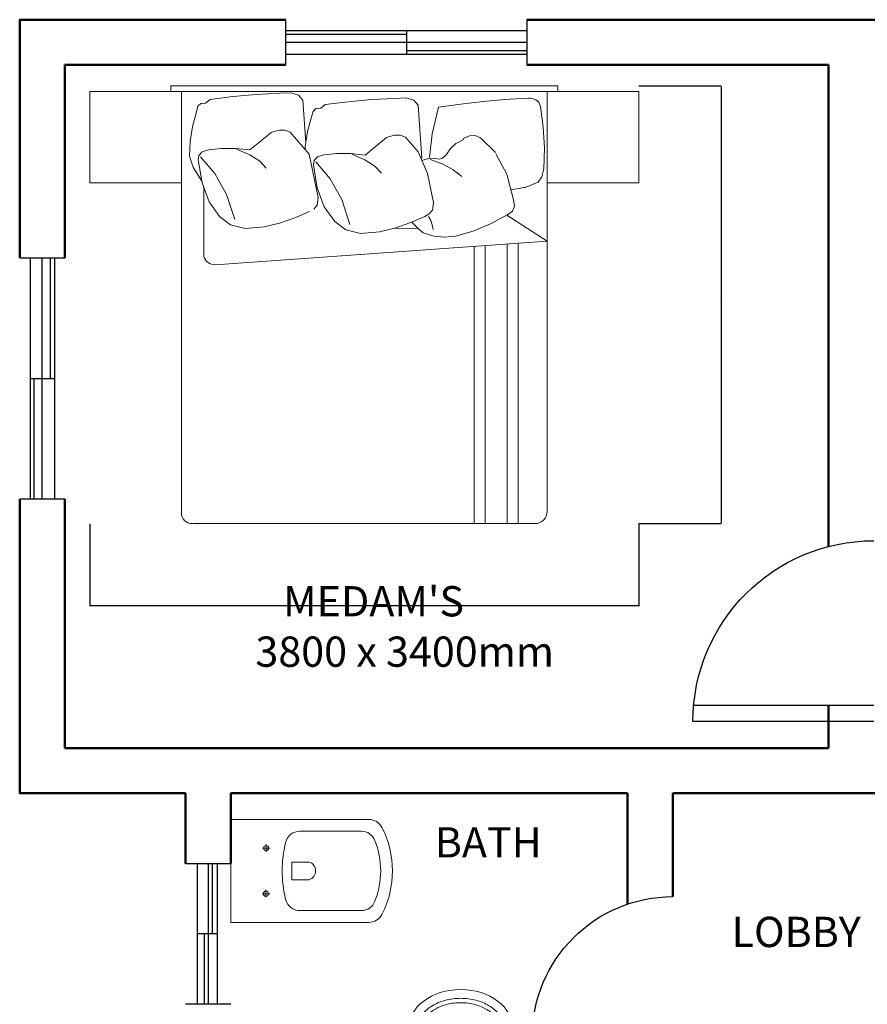
# Model space of a CAD drawing. Units: millimetres. Extents: x -857 to 54106, y -13666 to 13947.
# Tile 18 of 41: x 20195 to 24413, y 8304 to 13204. Entities that reach past the tile are written whole.
import ezdxf

# ---------------------------------------------------------------- set-up
doc = ezdxf.new("R2010")
doc.units = ezdxf.units.MM
for name, color, linetype, lineweight in [('A-ANNO-DIMS', 2, 'Continuous', 18), ('A-AREA-IDEN', 3, 'Continuous', 18), ('A-DOOR', 1, 'Continuous', 25), ('A-FLOR-FIXT', 8, 'Continuous', 18), ('A-FURN', 21, 'Continuous', 18), ('A-FURNITURE', 25, 'Continuous', 9), ('A-GLAZ', 4, 'Continuous', 25), ('A-SANITARY FITTINGS', 25, 'Continuous', 15), ('A-WALL', 7, 'Continuous', 50)]:
    doc.layers.add(name, color=color, linetype=linetype, lineweight=lineweight)
doc.styles.get("Standard").update_dxf_attribs({"font": 'arial.ttf'})
doc.dimstyles.new('ISO-25', dxfattribs={"dimtxt": 2.5, "dimasz": 2.5, "dimexe": 1.25, "dimexo": 0.625, "dimtad": 1, "dimtxsty": 'Standard', "dimcen": 2.5, "dimadec": 0, "dimazin": 0, "dimtfac": 1, "dimtmove": 0, "dimatfit": 3, "dimfxl": 1, "dimarcsym": 0})

# ---------------------------------------------------------------- blocks, each defined once
blk = doc.blocks.new('A$C06e6df2d')
at = {"layer": 'A-FURNITURE'}
for p, q in [((-73.01, 70.89), (-16.87, 70.89)), ((-70.22, 24.92), (-70.22, 70.89)), ((-68.43, 25.04), (-68.43, 70.89)), ((-64.83, 25.3), (-64.83, 70.89)), ((-63.04, 25.42), (-63.04, 70.89)), ((-75.01, 24.58), (-75.01, 68.89)), ((-15.01, 0), (-15.01, 69.09)), ((-75.01, 24.58), (-20.56, 28.42)), ((-18.69, 15.78), (-18.71, 27.06)), ((-68.39, 20.29), (-75.01, 24.58)), ((-75.01, 24.58), (-75.01, 0)), ((-65.73, 21.73), (-62.87, 22.91)), ((-62.87, 22.91), (-59.95, 23.77)), ((-59.95, 23.77), (-58.19, 23.92)), ((-58.19, 23.92), (-56.43, 23.73)), ((-56.43, 23.73), (-54.68, 23.22)), ((-56.16, 21.87), (-56.3, 22.64)), ((-54.68, 23.22), (-54.09, 22.72)), ((-54.09, 22.72), (-53.51, 22.17)), ((-50.02, 22.42), (-47.49, 23.05)), ((-47.49, 23.05), (-44.37, 23.33)), ((-44.37, 23.33), (-41.97, 22.72)), ((-41.97, 22.72), (-40.19, 21.34)), ((-68.53, 20.21), (-65.73, 21.73)), ((-55.9, 21.17), (-56.16, 21.87)), ((-55.54, 20.51), (-55.9, 21.17)), ((-54.92, 20.5), (-52.5, 21.58)), ((-49.77, 22.5), (-53.75, 22.43)), ((-53.51, 22.17), (-52.8, 21.44)), ((-52.5, 21.58), (-50.02, 22.42)), ((-41.32, 17.73), (-42.66, 21.83)), ((-40.19, 21.34), (-38.45, 18.93)), ((-33.6, 20.75), (-31.12, 21.59)), ((-31.12, 21.59), (-28.59, 22.22)), ((-28.59, 22.22), (-25.48, 22.5)), ((-25.48, 22.5), (-23.07, 21.9)), ((-22.42, 16.9), (-23.76, 21)), ((-23.07, 21.9), (-21.29, 20.51)), ((-69.62, 18.81), (-69.3, 19.62)), ((-69.3, 19.62), (-68.53, 20.21)), ((-56.34, 18.24), (-56.19, 19.49)), ((-56.19, 19.49), (-55.62, 20.16)), ((-55.62, 20.16), (-54.92, 20.5)), ((-36.02, 19.68), (-33.6, 20.75)), ((-21.29, 20.51), (-19.55, 18.1)), ((-69.5, 17.78), (-69.62, 18.81)), ((-68.39, 13.59), (-69.52, 17.98)), ((-55.37, 13.49), (-56.34, 18.24)), ((-38.45, 18.93), (-37.3, 15.81)), ((-37.44, 17.41), (-37.29, 18.66)), ((-37.29, 18.66), (-36.72, 19.34)), ((-19.55, 18.1), (-18.4, 14.98)), ((-69.05, 16.16), (-71.23, 15.78)), ((-39.4, 14.32), (-41.32, 17.73)), ((-35.98, 10.29), (-37.44, 17.41)), ((-20.5, 13.49), (-22.42, 16.9)), ((-73.5, 14.91), (-74.12, 14.04)), ((-71.64, 15.67), (-73.5, 14.91)), ((-71.25, 15.78), (-71.44, 15.74)), ((-37.3, 15.81), (-36.66, 12.07)), ((-18.4, 14.98), (-17.76, 11.24)), ((-16.95, 12.45), (-18.35, 14.73)), ((-74.12, 14.04), (-74.47, 12.68)), ((-66.57, 10.23), (-68.39, 13.59)), ((-61.02, 13.94), (-59.51, 12.79)), ((-53.83, 9.92), (-55.37, 13.49)), ((-47.81, 13.43), (-46.76, 12.26)), ((-37.06, 11.55), (-39.4, 14.32)), ((-18.16, 10.72), (-20.5, 13.49)), ((-74.47, 12.68), (-74.56, 9.28)), ((-59.51, 12.79), (-57.79, 11.86)), ((-57.79, 11.86), (-55.84, 11.15)), ((-54.44, 11.32), (-55.52, 11)), ((-46.76, 12.26), (-45.12, 11.25)), ((-36.79, 11.34), (-37.33, 10.73)), ((-36.66, 12.07), (-36.79, 11.34)), ((-28.91, 12.6), (-27.86, 11.44)), ((-27.86, 11.44), (-26.22, 10.43)), ((-16.34, 10.65), (-16.95, 12.45)), ((-64.09, 7.63), (-66.55, 10.02)), ((-58.52, 10.37), (-59.16, 9.35)), ((-58.11, 10.75), (-58.52, 10.37)), ((-57.7, 11.01), (-58.11, 10.75)), ((-57.28, 11.14), (-57.7, 11.01)), ((-56.4, 10.96), (-57.28, 11.14)), ((-55.52, 11), (-56.4, 10.96)), ((-56.14, 6.96), (-55.7, 10.85)), ((-54.44, 10.96), (-53.85, 2.28)), ((-51.75, 7.51), (-53.83, 9.92)), ((-45.15, 10.44), (-46.52, 9.32)), ((-42.78, 10.21), (-45.15, 10.44)), ((-45.12, 11.25), (-42.96, 10.31)), ((-40.52, 10.2), (-42.78, 10.21)), ((-38.37, 10.42), (-40.52, 10.2)), ((-37.33, 10.73), (-38.37, 10.42)), ((-32.85, 6.68), (-35.98, 10.29)), ((-26.22, 10.43), (-24.06, 9.48)), ((-18.43, 9.9), (-19.47, 9.59)), ((-17.89, 10.51), (-18.43, 9.9)), ((-17.76, 11.24), (-17.89, 10.51)), ((-16.43, 8.21), (-16.34, 10.65)), ((-74.56, 9.28), (-74.36, 5.88)), ((-60.04, 8.55), (-61.24, 7.96)), ((-59.16, 9.35), (-60.04, 8.55)), ((-47.98, 8.12), (-48.66, 7.55)), ((-46.52, 9.32), (-47.98, 8.12)), ((-35.72, 6.6), (-35.33, 9.04)), ((-35.43, 8.42), (-34.95, 1.45)), ((-35.33, 9.04), (-35.31, 9.52)), ((-27.62, 8.5), (-29.08, 7.29)), ((-26.26, 9.61), (-27.62, 8.5)), ((-23.88, 9.38), (-26.26, 9.61)), ((-21.62, 9.38), (-23.88, 9.38)), ((-19.47, 9.59), (-21.62, 9.38)), ((-16.82, 5.77), (-16.43, 8.21)), ((-63.18, 7.26), (-64.09, 7.63)), ((-62.27, 7.28), (-63.18, 7.26)), ((-61.35, 7.68), (-62.27, 7.28)), ((-61.24, 7.96), (-61.35, 7.68)), ((-57.17, 2.61), (-56.14, 6.96)), ((-50.88, 7.2), (-51.75, 7.51)), ((-50.02, 7.17), (-50.88, 7.2)), ((-49.15, 7.42), (-50.02, 7.17)), ((-48.66, 7.55), (-49.15, 7.42)), ((-36.37, 4.16), (-35.72, 6.6)), ((-31.98, 6.37), (-32.85, 6.68)), ((-30.25, 6.59), (-31.12, 6.34)), ((-29.76, 6.73), (-30.25, 6.59)), ((-29.08, 7.29), (-29.76, 6.73)), ((-74.36, 5.88), (-73.9, 2.49)), ((-31.12, 6.34), (-31.98, 6.37)), ((-17.47, 3.33), (-16.82, 5.77)), ((-37.09, 2.83), (-36.6, 3.27)), ((-36.6, 3.27), (-36.37, 4.16)), ((-17.71, 2.44), (-17.47, 3.33)), ((-73.9, 2.49), (-73.65, 1.74)), ((-73.65, 1.74), (-73.12, 1.41)), ((-68.06, 1.33), (-64.46, 1.68)), ((-64.46, 1.68), (-60.83, 2.11)), ((-60.83, 2.11), (-57.17, 2.61)), ((-53.85, 2.28), (-53.12, 1.45)), ((-46.17, 1.35), (-42.37, 1.69)), ((-42.37, 1.69), (-38.61, 2.15)), ((-38.61, 2.15), (-37.87, 2.73)), ((-37.87, 2.73), (-37.09, 2.83)), ((-19.71, 1.32), (-18.97, 1.91)), ((-18.97, 1.91), (-18.19, 2.01)), ((-18.19, 2.01), (-17.71, 2.44)), ((-76.74, 0), (-76.74, -0.9)), ((-13.27, 0), (-76.74, 0)), ((-71.96, 1.11), (-68.94, 1.26)), ((-68.94, 1.26), (-68.06, 1.33)), ((-53.12, 1.45), (-51.84, 1.07)), ((-51.84, 1.07), (-49.99, 1.14)), ((-49.99, 1.14), (-46.17, 1.35)), ((-34.95, 1.45), (-34.22, 0.63)), ((-34.22, 0.63), (-32.94, 0.25)), ((-32.94, 0.25), (-31.09, 0.31)), ((-31.09, 0.31), (-27.27, 0.52)), ((-27.27, 0.52), (-23.47, 0.86)), ((-23.47, 0.86), (-19.71, 1.32)), ((-13.27, -0.9), (-13.27, 0)), ((-13.27, -0.9), (-76.74, -0.9))]:
    blk.add_line(p, q, dxfattribs=at)
for points in [[(-75.01, 0), (-90.01, 0), (-90.01, 15.01), (-75.01, 15.01)], [(-15.01, 0), (0, 0), (0, 15.01), (-15.01, 15.01)]]:
    blk.add_lwpolyline(points, close=True, dxfattribs=at)
for centre, radius, start, end in [((-73.01, 68.89), 2, 90, 180), ((-16.8, 69.09), 1.8, 0, 90), ((-20.45, 26.63), 1.8, 13.7792, 93.47), ((-70.89, 13.81), 2, 99.8546, 112.1195), ((-72.06, 3.1), 2, 238.0354, 272.9353)]:
    blk.add_arc(centre, radius, start, end, dxfattribs=at)
blk = doc.blocks.new('A$C7d9d00ca')
at = {"layer": 'A-SANITARY FITTINGS'}
for p, q in [((0, 0), (-13.78, 0)), ((-13.78, -18.49), (-13.78, 0)), ((0, -18.49), (0, 0)), ((-10.42, -4.72), (-9.43, -4.72)), ((-9.94, -4.23), (-9.94, -5.23)), ((-3.36, -4.73), (-4.34, -4.73)), ((-3.84, -4.24), (-3.84, -5.24)), ((-12.2, -9.27), (-12.2, -17.48)), ((-1.57, -9.27), (-1.57, -17.48))]:
    blk.add_line(p, q, dxfattribs=at)
for points in [[(-8.08, -8.19), (-5.7, -8.19), (-5.7, -8.19), (-5.7, -10.48)], [(-8.08, -8.19), (-8.08, -10.48)]]:
    blk.add_lwpolyline(points, dxfattribs=at)
for centre in [(-9.94, -4.72), (-3.84, -4.73)]:
    blk.add_circle(centre, 0.342, dxfattribs=at)
for centre, radius, start, end in [((-10.24, -9.27), 1.97, 103.8652, 180), ((-6.89, -22.82), 15.93, 76.135, 103.8652), ((-3.54, -9.27), 1.97, 0.0003, 76.135), ((-6.89, -10.13), 1.24, 196.5098, 343.4902), ((-10.24, -17.48), 1.97, 180, 248.6555), ((-3.54, -17.48), 1.97, 291.3447, 0.0003), ((-11.81, -18.49), 1.97, 180, 242.8074), ((-6.89, -8.92), 11.16, 248.6555, 291.3447), ((-1.97, -18.49), 1.97, 297.1926, 0), ((-6.89, -8.92), 12.74, 242.8074, 297.1926)]:
    blk.add_arc(centre, radius, start, end, dxfattribs=at)
blk = doc.blocks.new('A$C0124305E')
at = {"layer": 'A-SANITARY FITTINGS'}
for p, q in [((-8.42, 16.01), (-0.8, 16.01)), ((-0.8, 7.08), (-0.8, 16.01)), ((-5.66, 7.68), (-8, 5.88)), ((-7.73, 7.95), (-5.93, 5.62)), ((-4.31, 5.61), (-4.31, 7.96)), ((-3.91, 5.61), (-3.91, 7.96)), ((0, 7.08), (-4.99, 7.08)), ((0, 6.28), (-4.99, 6.28)), ((-0.8, -3.19), (-0.8, 6.28)), ((-8.42, -3.19), (-0.8, -3.19))]:
    blk.add_line(p, q, dxfattribs=at)
blk.add_lwpolyline([(-0.5, 16.01), (0, 16.01), (0, -3.19), (-0.5, -3.19)], close=True, dxfattribs=at)
for radius in [1.18, 0.885]:
    blk.add_circle((-6.83, 6.78), radius, dxfattribs=at)
at = {"layer": 'A-SANITARY FITTINGS', "extrusion": (0, 0, -1)}
blk.add_ellipse((-8.42, 6.41), major_axis=(0, 9.6), ratio=0.75, start_param=3.141593, end_param=6.283185, dxfattribs=at)
at = {"layer": 'A-SANITARY FITTINGS'}
for points, knots in [([(-2.82, 6.28), (-2.82, 5.74), (-2.87, 5.2), (-3.1, 3.74), (-3.37, 2.86), (-4.09, 1.28), (-4.55, 0.6), (-5.56, -0.5), (-6.12, -0.92), (-7.25, -1.45), (-7.83, -1.58), (-8.98, -1.59), (-9.55, -1.46), (-10.69, -0.93), (-11.25, -0.52), (-12.27, 0.57), (-12.72, 1.25), (-13.45, 2.82), (-13.72, 3.71), (-14.02, 5.56), (-14.05, 6.52), (-13.88, 8.41), (-13.67, 9.32), (-13.04, 10.99), (-12.62, 11.73), (-11.66, 12.96), (-11.12, 13.45), (-10, 14.13), (-9.43, 14.32), (-8.28, 14.45), (-7.7, 14.39), (-6.56, 14), (-5.99, 13.66), (-4.93, 12.71), (-4.44, 12.09), (-3.62, 10.62), (-3.3, 9.78), (-2.96, 8.29), (-2.87, 7.69), (-2.84, 7.08)], [1.58652, 1.58652, 1.58652, 1.58652, 1.780321, 1.780321, 2.120053, 2.120053, 2.459785, 2.459785, 2.799517, 2.799517, 3.139249, 3.139249, 3.478981, 3.478981, 3.818713, 3.818713, 4.158445, 4.158445, 4.498177, 4.498177, 4.837909, 4.837909, 5.177641, 5.177641, 5.517373, 5.517373, 5.857105, 5.857105, 6.196837, 6.196837, 6.536569, 6.536569, 6.876301, 6.876301, 7.216033, 7.216033, 7.555765, 7.555765, 7.774364, 7.774364, 7.774364, 7.774364]), ([(-3.62, 6.29), (-3.62, 5.76), (-3.67, 5.23), (-3.88, 3.96), (-4.1, 3.23), (-4.65, 1.95), (-4.98, 1.39), (-5.72, 0.46), (-6.12, 0.1), (-6.92, -0.44), (-7.32, -0.61), (-8.11, -0.8), (-8.5, -0.81), (-9.28, -0.69), (-9.68, -0.55), (-10.48, -0.08), (-10.89, 0.24), (-11.67, 1.13), (-12.05, 1.7), (-12.66, 3.01), (-12.9, 3.76), (-13.2, 5.38), (-13.25, 6.28), (-13.13, 8.02), (-12.95, 8.88), (-12.42, 10.42), (-12.06, 11.12), (-11.23, 12.25), (-10.77, 12.7), (-9.92, 13.26), (-9.53, 13.43), (-8.78, 13.62), (-8.41, 13.64), (-7.66, 13.54), (-7.28, 13.42), (-6.51, 13.02), (-6.12, 12.73), (-5.35, 11.95), (-4.97, 11.43), (-4.34, 10.23), (-4.08, 9.54), (-3.76, 8.24), (-3.67, 7.64), (-3.63, 7.03)], [1.58652, 1.58652, 1.58652, 1.58652, 1.790653, 1.790653, 2.093007, 2.093007, 2.384527, 2.384527, 2.676047, 2.676047, 2.967567, 2.967567, 3.259087, 3.259087, 3.550608, 3.550608, 3.842128, 3.842128, 4.155456, 4.155456, 4.468784, 4.468784, 4.806699, 4.806699, 5.144614, 5.144614, 5.482529, 5.482529, 5.820444, 5.820444, 6.099515, 6.099515, 6.378586, 6.378586, 6.657656, 6.657656, 6.936727, 6.936727, 7.23864, 7.23864, 7.540552, 7.540552, 7.774364, 7.774364, 7.774364, 7.774364])]:
    blk.add_open_spline(points, degree=3, knots=knots, dxfattribs=at)
blk = doc.blocks.new('DOOR-900')
blk.add_line((11417.3, 9811.5), (12317.3, 9811.5))
blk.add_arc((11417.3, 9811.5), 900, 0, 90)
blk = doc.blocks.new('DOOR-700')
blk.add_line((8245.5, 10779.2), (8245.5, 11479.2))
blk.add_arc((8245.5, 10779.2), 700, 90, 180)
blk = doc.blocks.new('WIN-1200')
for p, q in [((9371.3, 11750.2), (10571.3, 11750.2)), ((9371.3, 11731.7), (9971.3, 11731.7)), ((9971.3, 11750.2), (9971.3, 11630.7)), ((9371.3, 11691.7), (10571.3, 11691.7)), ((10571.3, 11630.7), (9371.3, 11630.7)), ((9971.3, 11651.7), (10571.3, 11651.7))]:
    blk.add_line(p, q)
for points in [[(9371.3, 11579.2), (9371.3, 11804.2)], [(10571.3, 11804.2), (10571.3, 11579.2)]]:
    blk.add_lwpolyline(points)
blk = doc.blocks.new('WIN-700')
for p, q in [((3626.3, 8304.2), (3626.3, 9004.2)), ((3679.8, 9004.2), (3679.8, 8304.2)), ((3699.8, 9004.2), (3699.8, 8654.2)), ((3724.4, 9004.2), (3724.4, 8304.2)), ((3724.4, 8654.2), (3626.3, 8654.2)), ((3659.8, 8654.2), (3659.8, 8304.2))]:
    blk.add_line(p, q)
for points in [[(3567.3, 9004.2), (3792.3, 9004.2)], [(3792.3, 8304.2), (3567.3, 8304.2)]]:
    blk.add_lwpolyline(points)
blk = doc.blocks.new('*D43')
at = {"layer": 'A-ANNO-DIMS', "color": 0, "lineweight": -2, "transparency": 16777216}
for p, q in [((20544, 10695.8), (20544, 10285.5)), ((23275.2, 10695.8), (23275.2, 10285.5)), ((23272.7, 10286.8), (20546.5, 10286.8))]:
    blk.add_line(p, q, dxfattribs=at)
at = {"layer": 'A-ANNO-DIMS', "color": 0, "transparency": 16777216}
for points in [[(20546.5, 10287.2), (20546.5, 10286.3), (20544, 10286.8)], [(23272.7, 10287.2), (23272.7, 10286.3), (23275.2, 10286.8)]]:
    blk.add_solid(points, dxfattribs=at)
at = {"layer": 'Defpoints', "color": 0, "transparency": 16777216}
for p in [(20544, 10696.4), (23275.2, 10696.4), (20544, 10286.8)]:
    blk.add_point(p, dxfattribs=at)
at = {"layer": 'A-ANNO-DIMS', "color": 0, "transparency": 16777216, "insert": (21909.6, 10288.7), "char_height": 2.5, "attachment_point": 5}
blk.add_mtext('DOUBLE BED 2731 TYP.', dxfattribs=at)
blk = doc.blocks.new('*D44')
at = {"layer": 'A-ANNO-DIMS', "color": 0, "lineweight": -2, "transparency": 16777216}
for p, q in [((23275.8, 12874.6), (23686.1, 12874.6)), ((23684.8, 12872.1), (23684.8, 10698.9)), ((23275.8, 10696.4), (23686.1, 10696.4))]:
    blk.add_line(p, q, dxfattribs=at)
at = {"layer": 'A-ANNO-DIMS', "color": 0, "transparency": 16777216}
for points in [[(23684.4, 12872.1), (23685.2, 12872.1), (23684.8, 12874.6)], [(23684.4, 10698.9), (23685.2, 10698.9), (23684.8, 10696.4)]]:
    blk.add_solid(points, dxfattribs=at)
at = {"layer": 'Defpoints', "color": 0, "transparency": 16777216}
for p in [(23275.2, 12874.6), (23275.2, 10696.4), (23684.8, 10696.4)]:
    blk.add_point(p, dxfattribs=at)
at = {"layer": 'A-ANNO-DIMS', "color": 0, "transparency": 16777216, "insert": (23682.9, 11785.5), "char_height": 2.5, "attachment_point": 5, "rotation": 90}
blk.add_mtext('2178 TYP.', dxfattribs=at)

msp = doc.modelspace()

# ---------------------------------------------------------------- linework, layer by layer
at = {"layer": 'A-DOOR'}
msp.add_line((24445.079, 9791.167), (23545.079, 9791.167), dxfattribs=at)
at = {"layer": 'A-WALL'}
for p, q in [((20420.079, 12018.868), (20420.079, 12979.231)), ((20420.079, 12979.231), (21519.317, 12979.231)), ((22719.317, 12979.231), (24220.079, 12979.231)), ((24220.079, 12979.231), (24220.079, 10582.588)), ((20420.079, 9579.231), (20420.079, 10818.868)), ((24220.079, 9791.167), (24220.079, 9579.231)), ((24220.079, 9579.231), (20420.079, 9579.231)), ((23220.079, 9354.231), (21245.079, 9354.231)), ((21245.079, 9354.231), (21245.079, 9004.231)), ((23220.079, 8802.942), (23220.079, 9354.231)), ((23445.079, 8840.088), (23445.079, 9354.231)), ((23445.079, 9354.231), (24645.079, 9354.231))]:
    msp.add_line(p, q, dxfattribs=at)
for points in [[(20195.079, 12018.868), (20195.079, 13204.231), (21519.317, 13204.231)], [(22719.317, 13204.231), (24852.246, 13204.231)], [(21020.079, 9004.231), (21020.079, 9354.231), (20195.079, 9354.231), (20195.079, 10818.868)]]:
    msp.add_lwpolyline(points, dxfattribs=at)

# ---------------------------------------------------------------- block references
at = {"layer": 'A-DOOR', "extrusion": (0, 0, -1), "zscale": -1}
msp.add_blockref('DOOR-900', (-35862.359, -100.315), dxfattribs=at)
at = {"layer": 'A-DOOR', "extrusion": (0, 0, -1), "zscale": -1, "rotation": 269.9999999999999}
msp.add_blockref('DOOR-700', (-34224.31, 16385.634), dxfattribs=at)
at = {"layer": 'A-FLOR-FIXT'}
for name, p, xscale, yscale, zscale, rotation in [('A$C7d9d00ca', (21245.079, 9224.133), 37.15841229138232, 37.15841229138232, 37.15841229138232, 89.99999999999999), ('A$C0124305E', (22215.607, 7954.231), 27.10344997005861, 27.10344997005861, 27.10344997005861, 270.0000000004072)]:
    msp.add_blockref(name, p, dxfattribs=dict(at, xscale=xscale, yscale=yscale, zscale=zscale, rotation=rotation))
at = {"layer": 'A-FURN', "xscale": 30.34175224512773, "yscale": 30.34175224512773, "zscale": 30.34175224512773, "rotation": 180}
msp.add_blockref('A$C06e6df2d', (20544.014, 12847.381), dxfattribs=at)
at = {"layer": 'A-GLAZ'}
for name, p in [('WIN-1200', (12147.976, 1400)), ('WIN-700', (17452.799, 0))]:
    msp.add_blockref(name, p, dxfattribs=at)
at = {"layer": 'A-GLAZ', "rotation": 90.00000000000063}
msp.add_blockref('WIN-1200', (31999.31, 1447.527), dxfattribs=at)

# ---------------------------------------------------------------- texts
at = {"layer": 'A-AREA-IDEN', "attachment_point": 1}
for s, insert, char_height in [("\\pxt0;   MEDAM'S\\P3800 x 3400mm", (21368.026, 10385.331), 150.48461), ('\\pxt0;BATH', (22260.536, 9185.607), 150.4846), ('\\pxt0;LOBBY', (23737.429, 8739.704), 150.48461)]:
    msp.add_mtext_dynamic_manual_height_columns(s, width=2554.22693, gutter_width=18810.576, heights=[2595.835], dxfattribs=dict(at, insert=insert, char_height=char_height))

# ---------------------------------------------------------------- dimensions: what is measured, and where the dimension line sits
at = {"layer": 'A-ANNO-DIMS'}
for base, p1, p2, angle, text, picture, middle in [((23684.826, 10696.421), (23275.154, 12874.64), (23275.154, 10696.421), 270, '<> TYP.', '*D44', (23682.924, 11785.53)), ((20544.014, 10286.75), (23275.154, 10696.421), (20544.014, 10696.421), 180, 'DOUBLE BED <> TYP.', '*D43', (21909.584, 10288.669))]:
    dim = msp.add_linear_dim(base=base, p1=p1, p2=p2, angle=angle, text=text, dimstyle='ISO-25', override={"dimdec": 0, "dimrnd": 0, "dimzin": 0, "dimlunit": 2}, dxfattribs=at)
    dim.commit()
    dim.dimension.update_dxf_attribs({"geometry": picture, "text_midpoint": middle})

doc.saveas('drawing.dxf')
